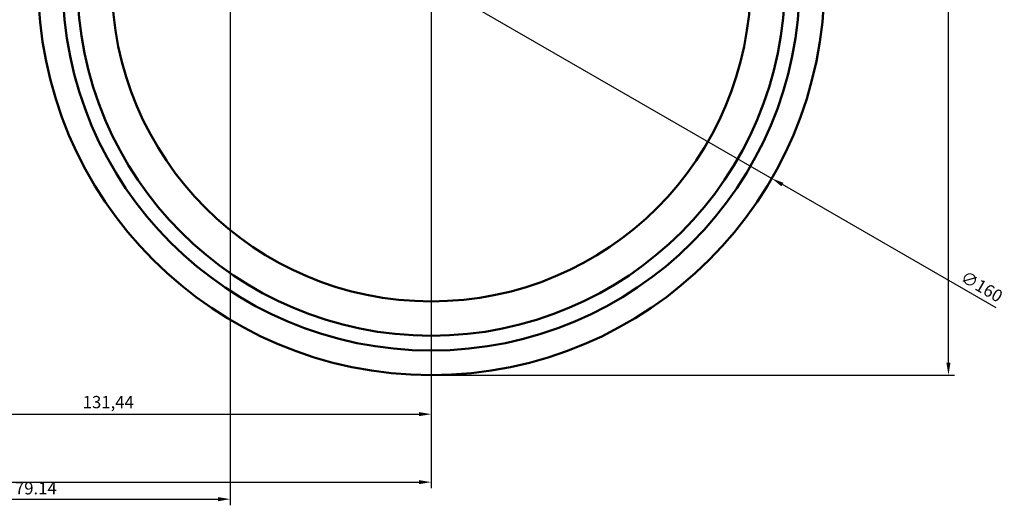
# Model space of a CAD drawing. Units: millimetres. Extents: x 1068 to 1546, y 1743 to 2032.
# Tile 6 of 9: x 1318 to 1519, y 1743 to 1842. Entities that reach past the tile are written whole.
import ezdxf

# ---------------------------------------------------------------- set-up
doc = ezdxf.new("R2010")
doc.units = ezdxf.units.MM
doc.layers.add('M-DIMS', color=2, linetype='Continuous', lineweight=25)
doc.layers.add('M-OUTL', color=7, linetype='Continuous', lineweight=50)
doc.styles.get("Standard").update_dxf_attribs({"font": 'arial.ttf'})
doc.dimstyles.new('ISO-25', dxfattribs={"dimtxt": 2.5, "dimasz": 2.5, "dimexe": 1.25, "dimexo": 0.625, "dimtad": 1, "dimtxsty": 'Standard', "dimcen": 2.5, "dimadec": 0, "dimazin": 0, "dimtfac": 1, "dimtmove": 0, "dimatfit": 3, "dimfxl": 1, "dimarcsym": 0})

# ---------------------------------------------------------------- blocks, each defined once
blk = doc.blocks.new('*D5')
at = {"layer": 'Defpoints', "color": 0, "transparency": 16777216}
for p in [(1177.23, 1849.76), (1402.23, 1849.76), (1402.23, 1747.98)]:
    blk.add_point(p, dxfattribs=at)
at = {"layer": 'M-DIMS', "color": 0, "lineweight": -2, "transparency": 16777216}
for p, q in [((1177.23, 1849.14), (1177.23, 1746.73)), ((1402.23, 1849.14), (1402.23, 1746.73)), ((1179.73, 1747.98), (1399.73, 1747.98))]:
    blk.add_line(p, q, dxfattribs=at)
at = {"layer": 'M-DIMS', "color": 0, "transparency": 16777216}
for points in [[(1179.73, 1748.39), (1179.73, 1747.56), (1177.23, 1747.98)], [(1399.73, 1748.39), (1399.73, 1747.56), (1402.23, 1747.98)]]:
    blk.add_solid(points, dxfattribs=at)
at = {"layer": 'M-DIMS', "color": 0, "transparency": 16777216, "insert": (1289.73, 1749.88), "char_height": 2.5, "attachment_point": 5}
blk.add_mtext('225', dxfattribs=at)
blk = doc.blocks.new('*D24')
at = {"layer": 'Defpoints', "color": 0, "transparency": 16777216}
for p in [(1270.79, 1850.31), (1402.23, 1850.31), (1402.23, 1761.81)]:
    blk.add_point(p, dxfattribs=at)
at = {"layer": 'M-DIMS', "color": 0, "lineweight": -2, "transparency": 16777216}
for p, q in [((1270.79, 1849.68), (1270.79, 1760.56)), ((1402.23, 1849.68), (1402.23, 1760.56)), ((1273.29, 1761.81), (1399.73, 1761.81))]:
    blk.add_line(p, q, dxfattribs=at)
at = {"layer": 'M-DIMS', "color": 0, "transparency": 16777216}
for points in [[(1273.29, 1762.23), (1273.29, 1761.4), (1270.79, 1761.81)], [(1399.73, 1762.23), (1399.73, 1761.4), (1402.23, 1761.81)]]:
    blk.add_solid(points, dxfattribs=at)
at = {"layer": 'M-DIMS', "color": 0, "transparency": 16777216, "insert": (1336.51, 1763.94), "char_height": 2.5, "attachment_point": 5}
blk.add_mtext('131,44', dxfattribs=at)
blk = doc.blocks.new('*D25')
at = {"layer": 'Defpoints', "color": 0, "transparency": 16777216}
for p in [(1376.21, 2002.95), (1507.48, 2002.95), (1402.23, 1769.76)]:
    blk.add_point(p, dxfattribs=at)
at = {"layer": 'M-DIMS', "color": 0, "lineweight": -2, "transparency": 16777216}
for p, q in [((1376.84, 2002.95), (1508.73, 2002.95)), ((1507.48, 1772.26), (1507.48, 2000.45)), ((1402.85, 1769.76), (1508.73, 1769.76))]:
    blk.add_line(p, q, dxfattribs=at)
at = {"layer": 'M-DIMS', "color": 0, "transparency": 16777216}
for points in [[(1507.06, 2000.45), (1507.89, 2000.45), (1507.48, 2002.95)], [(1507.06, 1772.26), (1507.89, 1772.26), (1507.48, 1769.76)]]:
    blk.add_solid(points, dxfattribs=at)
at = {"layer": 'M-DIMS', "color": 0, "transparency": 16777216, "insert": (1505.58, 1886.35), "char_height": 2.5, "attachment_point": 5, "rotation": 90}
blk.add_mtext('233.2', dxfattribs=at)
blk = doc.blocks.new('*D47')
at = {"layer": 'Defpoints', "color": 0, "transparency": 16777216}
for p in [(1361.34, 1946.14), (1282.2, 1868.65), (1361.34, 1744.51)]:
    blk.add_point(p, dxfattribs=at)
at = {"layer": 'M-DIMS', "color": 0, "lineweight": -2, "transparency": 16777216}
for p, q in [((1361.34, 1945.51), (1361.34, 1743.26)), ((1282.2, 1868.03), (1282.2, 1743.26)), ((1284.7, 1744.51), (1358.84, 1744.51))]:
    blk.add_line(p, q, dxfattribs=at)
at = {"layer": 'M-DIMS', "color": 0, "transparency": 16777216}
for points in [[(1284.7, 1744.93), (1284.7, 1744.1), (1282.2, 1744.51)], [(1358.84, 1744.93), (1358.84, 1744.1), (1361.34, 1744.51)]]:
    blk.add_solid(points, dxfattribs=at)
at = {"layer": 'M-DIMS', "color": 0, "transparency": 16777216, "insert": (1321.77, 1746.41), "char_height": 2.5, "attachment_point": 5}
blk.add_mtext('79.14', dxfattribs=at)
blk = doc.blocks.new('*D53')
at = {"layer": 'Defpoints', "color": 0, "transparency": 16777216}
for p in [(1332.93, 1889.74), (1471.52, 1809.79)]:
    blk.add_point(p, dxfattribs=at)
at = {"layer": 'M-DIMS', "color": 0, "lineweight": -2, "transparency": 16777216}
for p, q in [((1330.77, 1890.99), (1328.6, 1892.24)), ((1332.93, 1889.74), (1471.52, 1809.79)), ((1517.21, 1783.43), (1473.69, 1808.54))]:
    blk.add_line(p, q, dxfattribs=at)
at = {"layer": 'M-DIMS', "color": 0, "transparency": 16777216}
for points in [[(1330.98, 1891.35), (1330.56, 1890.63), (1332.93, 1889.74)], [(1473.9, 1808.9), (1473.48, 1808.18), (1471.52, 1809.79)]]:
    blk.add_solid(points, dxfattribs=at)
at = {"layer": 'M-DIMS', "color": 0, "transparency": 16777216, "insert": (1514.09, 1787.51), "char_height": 2.5, "attachment_point": 5, "rotation": 330.0197}
blk.add_mtext('∅160', dxfattribs=at)

msp = doc.modelspace()

# ---------------------------------------------------------------- linework, layer by layer
at = {"layer": 'M-OUTL'}
for radius in [80, 75, 72, 65]:
    msp.add_circle((1402.2281, 1849.7623), radius, dxfattribs=at)

# ---------------------------------------------------------------- dimensions: what is measured, and where the dimension line sits
at = {"layer": 'M-DIMS'}
dim = msp.add_linear_dim(base=(1507.4781, 2002.9476), p1=(1402.2281, 1769.7623), p2=(1376.2106, 2002.9476), angle=90, dimstyle='ISO-25', override={"dimdec": 1, "dimlfac": 1, "dimrnd": 0, "dimzin": 0, "dimdsep": 46, "dimlunit": 2}, dxfattribs=at)
dim.commit()
dim.dimension.update_dxf_attribs({"geometry": '*D25', "text_midpoint": (1505.5758, 1886.355)})
for base, p1, p2, override, picture, middle in [((1361.339, 1744.5123), (1282.1954, 1868.6519), (1361.339, 1946.1377), {"dimdec": 2, "dimlfac": 1, "dimrnd": 0, "dimzin": 0, "dimdsep": 46, "dimlunit": 2}, '*D47', (1321.7672, 1746.4138)), ((1402.2281, 1747.9766), (1177.2281, 1849.7623), (1402.2281, 1849.7623), {"dimclrd": 0, "dimclre": 0, "dimclrt": 0}, '*D5', (1289.7281, 1749.8781)), ((1402.2281, 1761.8125), (1270.787, 1850.3085), (1402.2281, 1850.3085), {"dimclrd": 0, "dimclre": 0, "dimclrt": 0}, '*D24', (1336.5076, 1763.9399))]:
    dim = msp.add_linear_dim(base=base, p1=p1, p2=p2, dimstyle='ISO-25', override=override, dxfattribs=at)
    dim.commit()
    dim.dimension.update_dxf_attribs({"geometry": picture, "text_midpoint": middle})
dim = msp.add_diameter_dim_2p(p1=(1332.9323, 1889.7385), p2=(1471.5239, 1809.7862), dimstyle='ISO-25', override={"dimdec": 0, "dimlfac": 1, "dimrnd": 0, "dimzin": 0, "dimdsep": 46, "dimlunit": 2}, dxfattribs=at)
dim.commit()
dim.dimension.update_dxf_attribs({"geometry": '*D53', "text_midpoint": (1513.1014, 1785.8005), "dimtype": 163})

doc.saveas('drawing.dxf')
